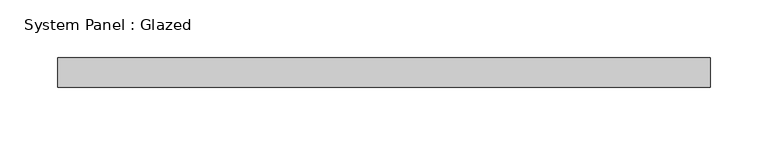
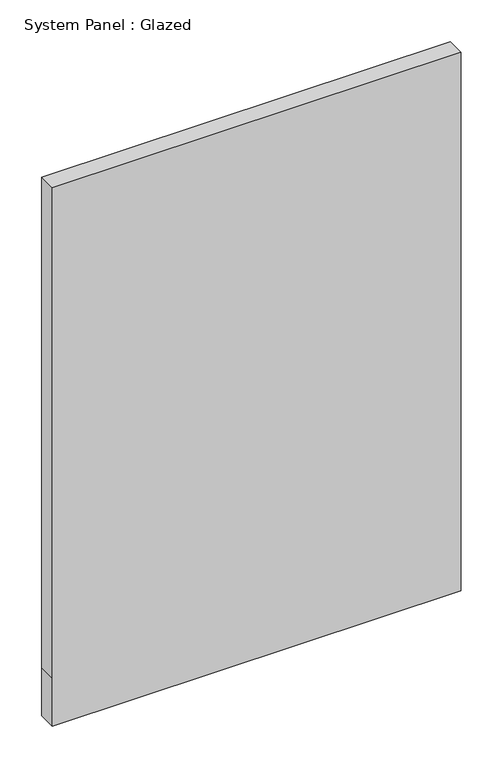
"""IFC4 building model written with IfcOpenShell, lengths in millimetres: plate geometry, System Panel : Glazed."""

from ifc_helpers import new_model, si_unit, frame, origin, place, context, project, spatial, polyline, outline, extrude, source, transform, mapped, element, save


def system_panel_glazed_71cd45ac(model_context):
    return source(origin(), model_context, "Body", "SweptSolid", [
        extrude(outline(polyline([(0.0, -282.575), (0.0, 282.575), (69.85, 282.575), (786.6309615, 282.575), (786.6309615, -282.575), (69.85, -282.575), (0.0, -282.575)])), frame((0.0, 19.05, 0.0), z_axis=(0.0, 1.0, 0.0), x_axis=(0.0, 0.0, 1.0)), (0.0, 0.0, 1.0), 25.4),
    ])


if __name__ == "__main__":
    model = new_model("IFC4")
    model_context = context("Model", 3, world=origin())
    ifc_project = project(units=[si_unit("LENGTHUNIT", "METRE", prefix="MILLI")], contexts=[model_context])
    site = spatial("IfcSite", under=ifc_project)
    building = spatial("IfcBuilding", under=site)
    placement = place(None, origin())
    system_panel_glazed_shape = system_panel_glazed_71cd45ac(model_context)
    element("IfcPlate", 1, ObjectType="System Panel : Glazed", at=placement, inside=building, context=model_context, shape_type="MappedRepresentation", body=[
        mapped(system_panel_glazed_shape, transform((0.0, 0.0, 0.0), x_axis=(1.0, 0.0, 0.0), y_axis=(0.0, 1.0, 0.0), z_axis=(0.0, 0.0, 1.0))),
    ])
    save(model, "model.ifc")

# Revit data of these elements
# Type "System Panel : Glazed"
#   Construction Type Id = "GSP4R"
#   Analytic Construction = "1/8 in Pilkington single glazing"
#   Visual Light Transmittance = 0.9
#   Solar Heat Gain Coefficient = 0.86
#   Heat Transfer Coefficient (U) = 1.18115 BTU/(h·ft²·°F)
#   Define Thermal Properties by = 1
# Element 1 (IfcPlate, "System Panel : Glazed")
#   Materials on its faces: "Glass"
# Materials
#   "Glass": class "Glass", colour RGB 0 128 192, transparency 0.75, Description = "Soda Lime Glass", Cost = 0
